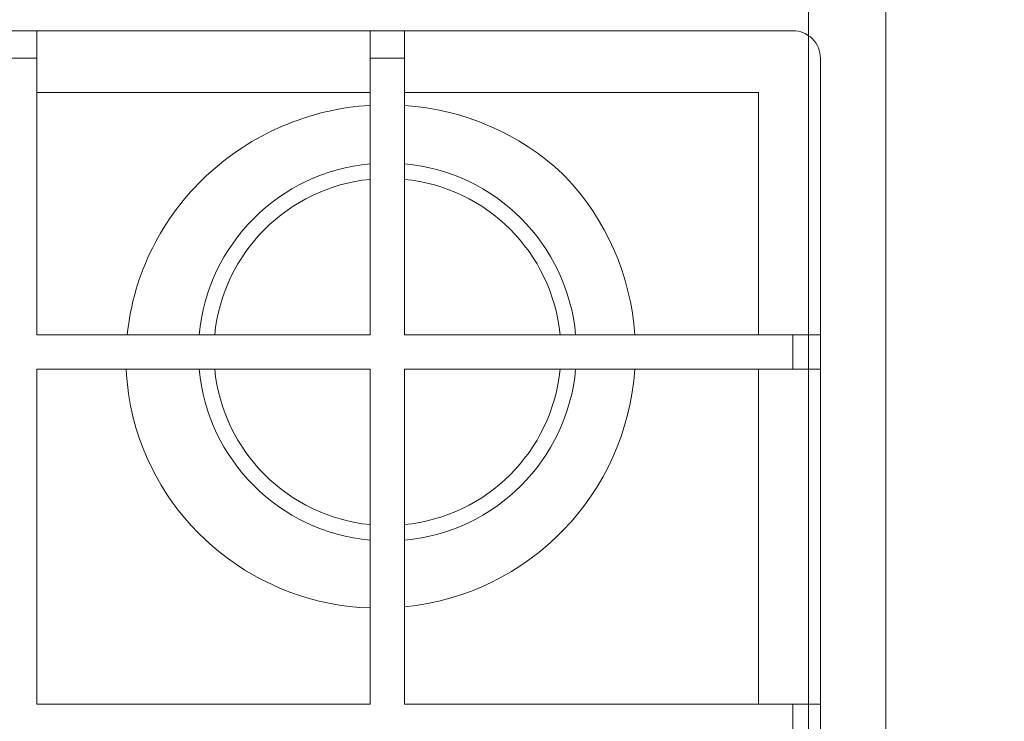
# Model space of a CAD drawing. Units: inches. Extents: x -1198 to -69, y -512 to 437.
# Tile 32 of 50: x -635.36 to -622.66, y 171.46 to 180.52. Entities that reach past the tile are written whole.
import ezdxf

# ---------------------------------------------------------------- set-up
doc = ezdxf.new("R2010")
doc.units = ezdxf.units.IN
doc.header["$MEASUREMENT"] = 0
for name, color, linetype, lineweight in [('0_Pen_No__7', 7, 'Continuous', 18), ('A-ANNO-DIMS', 2, 'Continuous', 18), ('A-EQPM', 60, 'Continuous', 18)]:
    doc.layers.add(name, color=color, linetype=linetype, lineweight=lineweight)
doc.styles.get("Standard").update_dxf_attribs({"font": 'arial.ttf'})
doc.dimstyles.get("Standard").update_dxf_attribs({"dimtxt": 6, "dimasz": 6, "dimexe": 0.18, "dimexo": 0.0625, "dimgap": 0.09, "dimtad": 0, "dimtih": 1, "dimtoh": 1, "dimdec": 0, "dimzin": 0, "dimdsep": 46, "dimlunit": 4, "dimtxsty": 'Standard', "dimblk": 'OBLIQUE', "dimcen": 0.09, "dimadec": 0, "dimazin": 0, "dimtfac": 1, "dimtdec": 0, "dimtofl": 0, "dimtmove": 0, "dimatfit": 3, "dimfxl": 1, "dimtolj": 1, "dimtzin": 0, "dimarcsym": 0})

# ---------------------------------------------------------------- blocks, each defined once
blk = doc.blocks.new('new block')
at = {"layer": '0_Pen_No__7'}
for p, q in [((-328.59, 344.07), (-328.59, 355.33)), ((-317.33, 344.07), (-317.33, 234.26)), ((-328.59, 234.26), (-328.59, 223)), ((-190.06, 143.6), (-80.82, 143.6)), ((-201.32, 132.33), (-190.06, 132.33)), ((-80.82, 132.33), (-69.55, 132.33))]:
    blk.add_line(p, q, dxfattribs=at)
for points in [[(-354.49, 596.91), (481.18, 596.91, -0.414214), (485.68, 592.4), (485.68, 99.11), (486.24, 99.11), (486.24, 95.73), (485.68, 95.73), (485.68, 4.5, -0.414214), (481.18, 0), (-354.49, 0, -0.414214), (-359, 4.5), (-359, 95.73), (-359.56, 95.73), (-359.56, 99.11), (-359, 99.11), (-359, 592.4, -0.414214)], [(464.28, 132.33), (464.28, 567.06, 0.414214), (455.27, 576.07), (-328.59, 576.07, 0.414214), (-337.6, 567.06), (-337.6, 132.33, 0.414214), (-328.59, 123.32), (455.27, 123.32, 0.414214)]]:
    blk.add_lwpolyline(points, format="xyb", close=True, dxfattribs=at)
for points in [[(-333.7, 12.95), (460.3, 12.95), (460.3, 570.44), (-333.7, 570.44)], [(-80.82, 234.26), (-80.82, 344.07), (-190.06, 344.07), (-190.06, 234.26)]]:
    blk.add_lwpolyline(points, close=True, dxfattribs=at)
for points in [[(-337.6, 234.26), (-201.32, 234.26), (-201.32, 344.07), (-337.6, 344.07)], [(-201.32, 123.32), (-201.32, 223), (-337.6, 223)], [(-317.33, 223), (-317.33, 143.6), (-201.32, 143.6)], [(-80.82, 123.32), (-80.82, 223), (-190.06, 223), (-190.06, 123.32)], [(-190.06, 147.76), (-188.21, 147.89), (-186.35, 148.06), (-184.5, 148.28), (-182.66, 148.53), (-180.82, 148.83), (-178.99, 149.16), (-177.16, 149.53), (-175.35, 149.94), (-173.54, 150.39), (-171.74, 150.88), (-169.96, 151.41), (-168.18, 151.98), (-166.42, 152.58), (-164.68, 153.23), (-162.94, 153.9), (-161.22, 154.62), (-159.52, 155.37), (-157.84, 156.16), (-156.17, 156.99), (-154.52, 157.85), (-152.89, 158.75), (-151.28, 159.68), (-149.69, 160.65), (-148.12, 161.65), (-146.57, 162.68), (-145.04, 163.75), (-143.54, 164.85), (-142.07, 165.98), (-140.61, 167.15), (-139.19, 168.34), (-137.79, 169.57), (-136.42, 170.82), (-135.07, 172.11), (-133.75, 173.43), (-132.47, 174.77), (-131.21, 176.14), (-129.98, 177.54), (-128.79, 178.97), (-127.62, 180.42), (-126.49, 181.9), (-125.39, 183.4), (-124.33, 184.93), (-123.3, 186.48), (-122.3, 188.05), (-121.34, 189.64), (-120.42, 191.26), (-119.53, 192.89), (-118.68, 194.55), (-117.87, 196.22), (-117.09, 197.91), (-116.36, 199.62), (-115.66, 201.35), (-115, 203.09), (-114.38, 204.84), (-113.8, 206.61), (-113.26, 208.39), (-112.76, 210.19), (-112.31, 211.99), (-111.89, 213.81), (-111.52, 215.63), (-111.19, 217.46), (-110.9, 219.3), (-110.65, 221.15), (-110.45, 222.99)]]:
    blk.add_lwpolyline(points, dxfattribs=at)
for centre, radius, start, end in [((-193.03, 228.66), 83.93, 95.6702, 176.1745), ((-192.8, 229.51), 83.08, 14.6793, 88.1082), ((-195.69, 228.63), 61.94, 95.2168, 174.7836), ((-195.69, 228.63), 61.94, 5.2164, 84.7832), ((-195.69, 228.63), 56.88, 95.6822, 174.3178), ((-195.69, 228.63), 56.88, 5.6822, 84.3178), ((-130.93, 245.73), 19.12, 13.6505, 14.6398), ((-191.8, 230.95), 81.75, 2.3165, 13.6452), ((-193.43, 228.67), 83.53, 183.8969, 223.6071), ((-195.69, 228.63), 61.94, 185.2164, 264.7832), ((-195.69, 228.63), 56.88, 185.6822, 264.3178), ((-195.69, 228.63), 61.94, 275.2168, 354.7836), ((-195.69, 228.63), 56.88, 275.6822, 354.3178), ((-239.43, 184.87), 20.01, 223.6326, 226.8635), ((-195.64, 231.83), 84.22, 226.9693, 266.1293)]:
    blk.add_arc(centre, radius, start, end, dxfattribs=at)
blk = doc.blocks.new('_Oblique')
at = {"color": 0, "linetype": 'ByBlock', "lineweight": -2}
blk.add_line((-0.5, -0.5), (0.5, 0.5), dxfattribs=at)
blk = doc.blocks.new('*D56')
at = {"layer": 'A-ANNO-DIMS', "color": 0, "lineweight": -2, "ltscale": 10, "transparency": 16777216}
for p, q in [((-618.339, 257.228), (-603.822, 257.228)), ((-604.002, 257.228), (-604.002, 212.422)), ((-604.002, 161.228), (-604.002, 206.033)), ((-618.339, 161.228), (-603.822, 161.228))]:
    blk.add_line(p, q, dxfattribs=at)
at = {"layer": 'DEFPOINTS', "color": 0, "ltscale": 10, "transparency": 16777216}
for p in [(-618.402, 257.228), (-604.002, 257.228), (-618.402, 161.228)]:
    blk.add_point(p, dxfattribs=at)
at = {"layer": 'A-ANNO-DIMS', "color": 0, "lineweight": -2, "ltscale": 10, "transparency": 16777216, "xscale": 6, "yscale": 6, "zscale": 6}
for p, rotation in [((-604.002, 257.228), 90), ((-604.002, 161.228), 270)]:
    blk.add_blockref('_Oblique', p, dxfattribs=dict(at, rotation=rotation))
at = {"layer": 'A-ANNO-DIMS', "color": 0, "ltscale": 10, "transparency": 16777216, "insert": (-604.002, 209.228), "char_height": 6, "attachment_point": 5}
blk.add_mtext('\\A1;COUNTER 96 TYP.', dxfattribs=at)

msp = doc.modelspace()

# ---------------------------------------------------------------- block references
at = {"layer": 'A-EQPM', "xscale": 0.0393700787401575, "yscale": 0.0393700787401575, "zscale": 0.0393700787401575, "rotation": 180}
msp.add_blockref('new block', (-638.3186, 185.2277), dxfattribs=at)

# ---------------------------------------------------------------- dimensions: what is measured, and where the dimension line sits
at = {"layer": 'A-ANNO-DIMS', "ltscale": 10}
dim = msp.add_linear_dim(base=(-604.0019, 257.2277), p1=(-618.4019, 161.2277), p2=(-618.4019, 257.2277), angle=90, text='COUNTER <> TYP.', dimstyle='Standard', override={"dimdec": 0, "dimlfac": 1, "dimrnd": 0, "dimzin": 0, "dimdsep": 46, "dimlunit": 2}, dxfattribs=at)
dim.commit()
dim.dimension.update_dxf_attribs({"geometry": '*D56', "text_midpoint": (-604.0019, 209.2277)})

doc.saveas('drawing.dxf')
